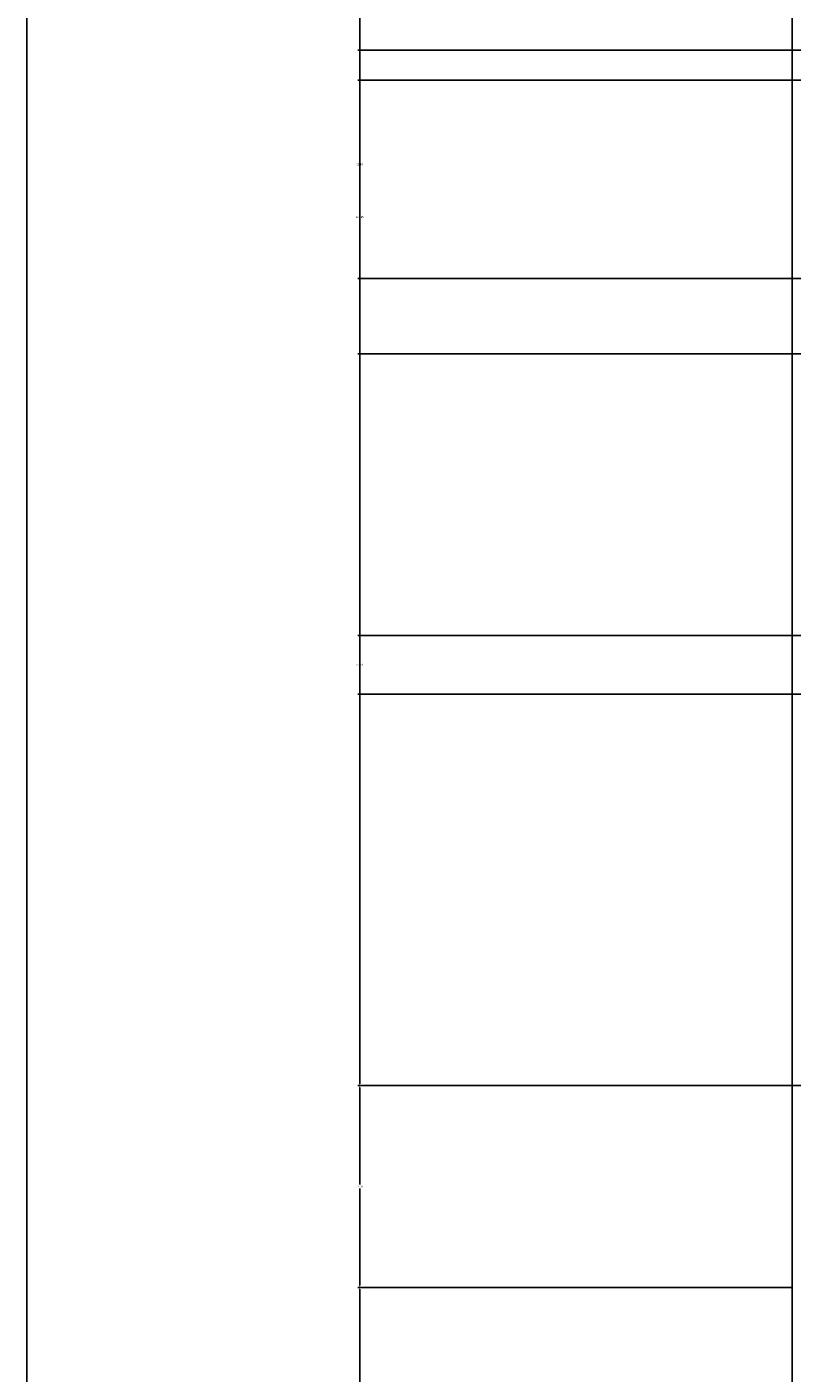
# Model space of a CAD drawing. Units: inches. Extents: x 1748 to 2382, y 1346 to 2284.
# Tile 17 of 26: x 1748 to 1822, y 1971 to 2102. Entities that reach past the tile are written whole.
import ezdxf

# ---------------------------------------------------------------- set-up
doc = ezdxf.new("R2010")
doc.units = ezdxf.units.IN
doc.layers.add('A-ANNO-DIMS', color=2, linetype='Continuous', lineweight=18)
doc.layers.add('A-ANNO-TTLB', color=7, linetype='Continuous', lineweight=25)
doc.styles.get("Standard").update_dxf_attribs({"font": 'arial.ttf'})
doc.dimstyles.get("Standard").update_dxf_attribs({"dimtxt": 0.18, "dimasz": 0.18, "dimexe": 0.18, "dimexo": 0.0625, "dimgap": 0.09, "dimtad": 0, "dimtih": 1, "dimtoh": 1, "dimdec": 4, "dimzin": 0, "dimdsep": 46, "dimtxsty": 'Standard', "dimcen": 0.09, "dimadec": 0, "dimazin": 0, "dimtfac": 1, "dimtdec": 4, "dimtofl": 0, "dimtmove": 0, "dimatfit": 3, "dimfxl": 1, "dimtolj": 1, "dimtzin": 0, "dimarcsym": 0})

# ---------------------------------------------------------------- blocks, each defined once
blk = doc.blocks.new('*D41')
at = {"layer": 'A-ANNO-DIMS', "color": 0, "lineweight": -2, "transparency": 16777216}
for p, q in [((1821.96, 1854.91), (1821.96, 2274.93)), ((1822.14, 2274.75), (1839.16, 2274.75)), ((1856.96, 2274.75), (1839.95, 2274.75)), ((1857.14, 1854.91), (1857.14, 2274.93))]:
    blk.add_line(p, q, dxfattribs=at)
at = {"layer": 'A-ANNO-DIMS', "color": 0, "transparency": 16777216}
for points in [[(1822.14, 2274.78), (1822.14, 2274.72), (1821.96, 2274.75)], [(1856.96, 2274.78), (1856.96, 2274.72), (1857.14, 2274.75)]]:
    blk.add_solid(points, dxfattribs=at)
at = {"layer": 'Defpoints', "color": 0, "transparency": 16777216}
for p in [(1857.14, 2274.75), (1821.96, 1854.85), (1857.14, 1854.85)]:
    blk.add_point(p, dxfattribs=at)
at = {"layer": 'A-ANNO-DIMS', "color": 0, "transparency": 16777216, "insert": (1839.55, 2274.75), "char_height": 0.18, "attachment_point": 5}
blk.add_mtext('\\A1;35.18', dxfattribs=at)
blk = doc.blocks.new('*D45')
at = {"layer": 'A-ANNO-DIMS', "color": 0, "lineweight": -2, "transparency": 16777216}
for p, q in [((1821.9, 2232.85), (1779.88, 2232.85)), ((1780.06, 2232.67), (1780.06, 2116.07)), ((1780.06, 1999.11), (1780.06, 2115.71)), ((1865.4, 1998.93), (1779.88, 1998.93))]:
    blk.add_line(p, q, dxfattribs=at)
at = {"layer": 'A-ANNO-DIMS', "color": 0, "transparency": 16777216}
for points in [[(1780.03, 2232.67), (1780.09, 2232.67), (1780.06, 2232.85)], [(1780.03, 1999.11), (1780.09, 1999.11), (1780.06, 1998.93)]]:
    blk.add_solid(points, dxfattribs=at)
at = {"layer": 'Defpoints', "color": 0, "transparency": 16777216}
for p in [(1780.06, 2232.85), (1821.96, 2232.85), (1865.46, 1998.93)]:
    blk.add_point(p, dxfattribs=at)
at = {"layer": 'A-ANNO-DIMS', "color": 0, "transparency": 16777216, "insert": (1780.06, 2115.89), "char_height": 0.18, "attachment_point": 5}
blk.add_mtext('\\A1;233.9', dxfattribs=at)
blk = doc.blocks.new('*D57')
at = {"layer": 'A-ANNO-DIMS', "color": 0, "lineweight": -2, "transparency": 16777216}
for p, q in [((2288.4, 2099.35), (1779.88, 2099.35)), ((1780.06, 2099.17), (1780.06, 2088.46)), ((1780.06, 2077.38), (1780.06, 2088.09)), ((2288.4, 2077.2), (1779.88, 2077.2))]:
    blk.add_line(p, q, dxfattribs=at)
at = {"layer": 'A-ANNO-DIMS', "color": 0, "transparency": 16777216}
for points in [[(1780.03, 2099.17), (1780.09, 2099.17), (1780.06, 2099.35)], [(1780.03, 2077.38), (1780.09, 2077.38), (1780.06, 2077.2)]]:
    blk.add_solid(points, dxfattribs=at)
at = {"layer": 'Defpoints', "color": 0, "transparency": 16777216}
for p in [(1780.06, 2099.35), (2288.46, 2099.35), (2288.46, 2077.2)]:
    blk.add_point(p, dxfattribs=at)
at = {"layer": 'A-ANNO-DIMS', "color": 0, "transparency": 16777216, "insert": (1780.06, 2088.28), "char_height": 0.18, "attachment_point": 5}
blk.add_mtext('\\A1;22.15', dxfattribs=at)
blk = doc.blocks.new('*D63')
at = {"layer": 'A-ANNO-DIMS', "color": 0, "lineweight": -2, "transparency": 16777216}
for p, q in [((2253.72, 2042.57), (1779.88, 2042.57)), ((1780.06, 2042.39), (1780.06, 2039.92)), ((1780.06, 2037.08), (1780.06, 2039.55)), ((2253.72, 2036.9), (1779.88, 2036.9))]:
    blk.add_line(p, q, dxfattribs=at)
at = {"layer": 'A-ANNO-DIMS', "color": 0, "transparency": 16777216}
for points in [[(1780.03, 2042.39), (1780.09, 2042.39), (1780.06, 2042.57)], [(1780.03, 2037.08), (1780.09, 2037.08), (1780.06, 2036.9)]]:
    blk.add_solid(points, dxfattribs=at)
at = {"layer": 'Defpoints', "color": 0, "transparency": 16777216}
for p in [(1780.06, 2042.57), (2253.78, 2042.57), (2253.78, 2036.9)]:
    blk.add_point(p, dxfattribs=at)
at = {"layer": 'A-ANNO-DIMS', "color": 0, "transparency": 16777216, "insert": (1780.06, 2039.74), "char_height": 0.18, "attachment_point": 5}
blk.add_mtext('\\A1;5.673', dxfattribs=at)
blk = doc.blocks.new('*D69')
at = {"layer": 'A-ANNO-DIMS', "color": 0, "lineweight": -2, "transparency": 16777216}
for p, q in [((1865.4, 1998.93), (1779.88, 1998.93)), ((1780.06, 1998.75), (1780.06, 1989.32)), ((1780.06, 1979.53), (1780.06, 1988.96)), ((1821.9, 1979.35), (1779.88, 1979.35))]:
    blk.add_line(p, q, dxfattribs=at)
at = {"layer": 'A-ANNO-DIMS', "color": 0, "transparency": 16777216}
for points in [[(1780.03, 1998.75), (1780.09, 1998.75), (1780.06, 1998.93)], [(1780.03, 1979.53), (1780.09, 1979.53), (1780.06, 1979.35)]]:
    blk.add_solid(points, dxfattribs=at)
at = {"layer": 'Defpoints', "color": 0, "transparency": 16777216}
for p in [(1780.06, 1998.93), (1865.46, 1998.93), (1821.96, 1979.35)]:
    blk.add_point(p, dxfattribs=at)
at = {"layer": 'A-ANNO-DIMS', "color": 0, "transparency": 16777216, "insert": (1780.06, 1989.14), "char_height": 0.18, "attachment_point": 5}
blk.add_mtext('\\A1;19.58', dxfattribs=at)
blk = doc.blocks.new('*D72')
at = {"layer": 'A-ANNO-DIMS', "color": 0, "lineweight": -2, "transparency": 16777216}
for p, q in [((1821.9, 1979.35), (1779.88, 1979.35)), ((1780.06, 1979.17), (1780.06, 1966.25)), ((1780.06, 1952.97), (1780.06, 1965.89)), ((1821.9, 1952.79), (1779.88, 1952.79))]:
    blk.add_line(p, q, dxfattribs=at)
at = {"layer": 'A-ANNO-DIMS', "color": 0, "transparency": 16777216}
for points in [[(1780.03, 1979.17), (1780.09, 1979.17), (1780.06, 1979.35)], [(1780.03, 1952.97), (1780.09, 1952.97), (1780.06, 1952.79)]]:
    blk.add_solid(points, dxfattribs=at)
at = {"layer": 'Defpoints', "color": 0, "transparency": 16777216}
for p in [(1780.06, 1979.35), (1821.96, 1979.35), (1821.96, 1952.79)]:
    blk.add_point(p, dxfattribs=at)
at = {"layer": 'A-ANNO-DIMS', "color": 0, "transparency": 16777216, "insert": (1780.06, 1966.07), "char_height": 0.18, "attachment_point": 5}
blk.add_mtext('\\A1;26.56', dxfattribs=at)
blk = doc.blocks.new('*D76')
at = {"layer": 'A-ANNO-DIMS', "color": 0, "lineweight": -2, "transparency": 16777216}
for p, q in [((2025.9, 2096.43), (1779.88, 2096.43)), ((1780.06, 2096.25), (1780.06, 2083.35)), ((1780.06, 2070.08), (1780.06, 2082.98)), ((2025.9, 2069.9), (1779.88, 2069.9))]:
    blk.add_line(p, q, dxfattribs=at)
at = {"layer": 'A-ANNO-DIMS', "color": 0, "transparency": 16777216}
for points in [[(1780.03, 2096.25), (1780.09, 2096.25), (1780.06, 2096.43)], [(1780.03, 2070.08), (1780.09, 2070.08), (1780.06, 2069.9)]]:
    blk.add_solid(points, dxfattribs=at)
at = {"layer": 'Defpoints', "color": 0, "transparency": 16777216}
for p in [(1780.06, 2096.43), (2025.96, 2096.43), (2025.96, 2069.9)]:
    blk.add_point(p, dxfattribs=at)
at = {"layer": 'A-ANNO-DIMS', "color": 0, "transparency": 16777216, "insert": (1780.06, 2083.16), "char_height": 0.18, "attachment_point": 5}
blk.add_mtext('\\A1;26.535', dxfattribs=at)

msp = doc.modelspace()

# ---------------------------------------------------------------- linework, layer by layer
at = {"layer": 'A-ANNO-TTLB'}
msp.add_lwpolyline([(1747.8112, 2284.3704), (2382.1361, 2284.3704), (2382.1361, 1346.4899), (1747.8112, 1346.4899)], close=True, dxfattribs=at)

# ---------------------------------------------------------------- dimensions: what is measured, and where the dimension line sits
at = {"layer": 'A-ANNO-DIMS'}
dim = msp.add_linear_dim(base=(1857.1427, 2274.7497), p1=(1821.9607, 1854.8497), p2=(1857.1427, 1854.8497), dimstyle='Standard', override={"dimdec": 2, "dimlfac": 1, "dimrnd": 0, "dimzin": 0, "dimdsep": 46, "dimlunit": 2}, dxfattribs=at)
dim.commit()
dim.dimension.update_dxf_attribs({"geometry": '*D41', "text_midpoint": (1839.5517, 2274.7497)})
for base, p1, p2, override, picture, middle in [((1780.0607, 2232.8497), (1865.4607, 1998.93), (1821.9607, 2232.8497), {"dimdec": 1, "dimlfac": 1, "dimrnd": 0, "dimzin": 0, "dimdsep": 46, "dimlunit": 2}, '*D45', (1780.0607, 2115.8898)), ((1780.0607, 2099.3497), (2288.4607, 2077.2008), (2288.4607, 2099.3497), {"dimdec": 2, "dimlfac": 1, "dimrnd": 0, "dimzin": 0, "dimdsep": 46, "dimlunit": 2}, '*D57', (1780.0607, 2088.2752)), ((1780.06066, 2096.4326), (2025.96066, 2069.89715), (2025.96066, 2096.4326), {"dimdec": 3, "dimlfac": 1, "dimrnd": 0, "dimzin": 0, "dimdsep": 46, "dimlunit": 2}, '*D76', (1780.06066, 2083.16488)), ((1780.0607, 2042.573), (2253.7809, 2036.9), (2253.7809, 2042.573), {"dimdec": 3, "dimlfac": 1, "dimrnd": 0, "dimzin": 0, "dimdsep": 46, "dimlunit": 2}, '*D63', (1780.0607, 2039.7365)), ((1780.0607, 1998.93), (1821.9607, 1979.3497), (1865.4607, 1998.93), {"dimdec": 2, "dimlfac": 1, "dimrnd": 0, "dimzin": 0, "dimdsep": 46, "dimlunit": 2}, '*D69', (1780.0607, 1989.1398)), ((1780.0607, 1979.3497), (1821.9607, 1952.7922), (1821.9607, 1979.3497), {"dimdec": 2, "dimlfac": 1, "dimrnd": 0, "dimzin": 0, "dimdsep": 46, "dimlunit": 2}, '*D72', (1780.0607, 1966.0709))]:
    dim = msp.add_linear_dim(base=base, p1=p1, p2=p2, angle=90, dimstyle='Standard', override=override, dxfattribs=at)
    dim.commit()
    dim.dimension.update_dxf_attribs({"geometry": picture, "text_midpoint": middle})

doc.saveas('drawing.dxf')
